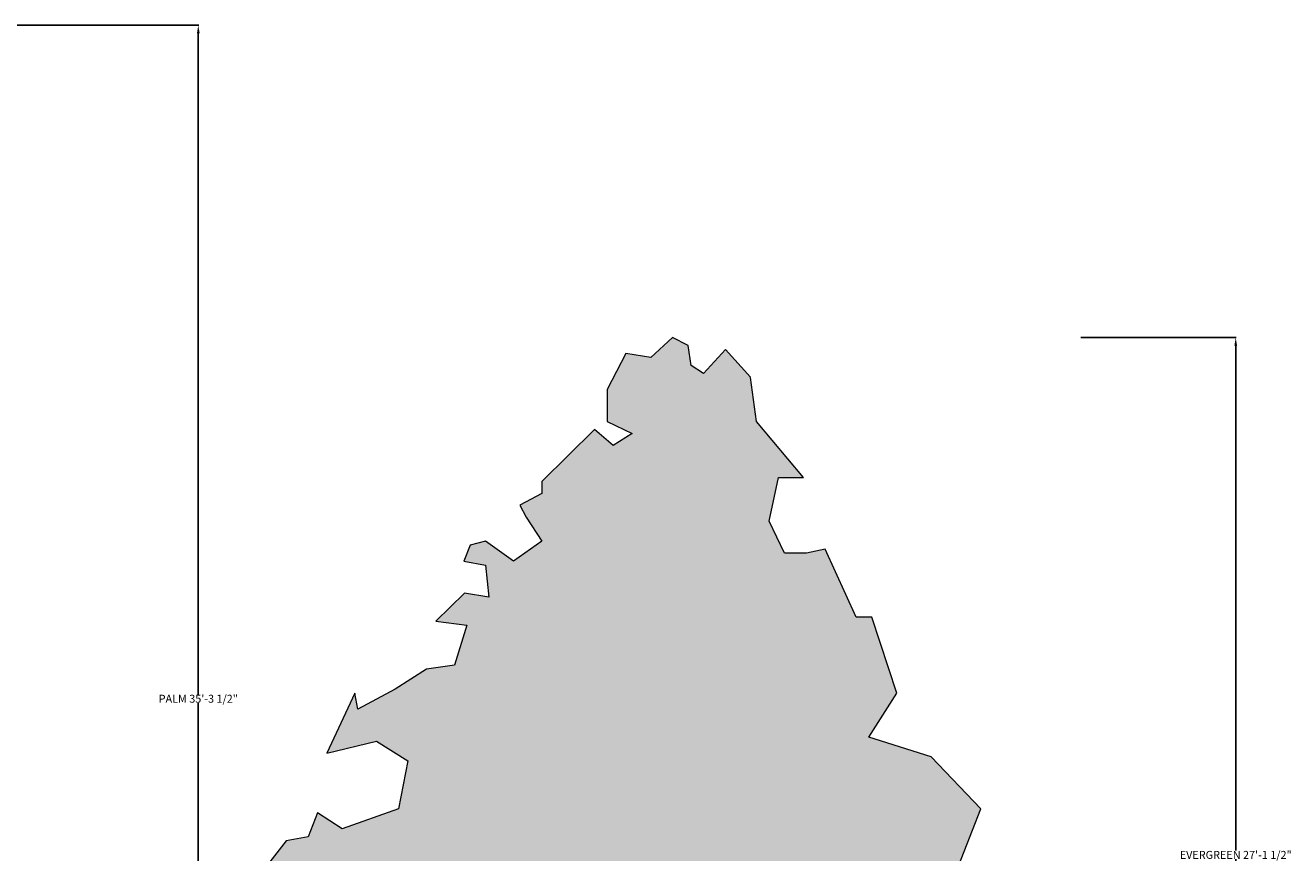
# Model space of a CAD drawing. Units: inches. Extents: x 481 to 2783, y 1975 to 3327.
# Tile 13 of 13: x 2331 to 2729, y 2286 to 2547. Entities that reach past the tile are written whole.
import ezdxf

# ---------------------------------------------------------------- set-up
doc = ezdxf.new("R2010")
doc.units = ezdxf.units.IN
doc.header["$MEASUREMENT"] = 0
doc.layers.add('A-ANNO-DIMS', color=50, linetype='Continuous', lineweight=18)
doc.layers.add('L-PLNT', color=7, linetype='Continuous', lineweight=13)
doc.layers.add('L-PLNT-PATT', color=116, linetype='Continuous', lineweight=13, true_color=0x136734)
doc.styles.get("Standard").update_dxf_attribs({"font": 'arial.ttf'})
doc.dimstyles.get("Standard").update_dxf_attribs({"dimtxt": 2.5, "dimasz": 2.5, "dimexe": 0.18, "dimexo": 0.0625, "dimgap": 0.09, "dimtad": 0, "dimtih": 1, "dimtoh": 1, "dimzin": 0, "dimdsep": 46, "dimlunit": 3, "dimtxsty": 'Standard', "dimcen": 0.09, "dimadec": 0, "dimazin": 0, "dimtfac": 1, "dimtofl": 0, "dimtmove": 0, "dimatfit": 3, "dimfxl": 1, "dimtolj": 1, "dimtzin": 0, "dimarcsym": 0})

# ---------------------------------------------------------------- blocks, each defined once
blk = doc.blocks.new('Tree - type 3 evergreen elevation')
for points in [[(22.0124, 137.721), (18.5475, 141.5624), (15.5282, 138.2446), (13.8028, 139.3505), (13.3714, 142.1153), (11.2148, 143.2214), (8.1954, 140.4564), (4.7447, 141.0094), (2.1567, 136.0326), (2.1567, 131.6088), (5.6074, 129.9499), (3.0193, 128.2909), (0.4313, 130.5029), (-6.9015, 123.3141), (-6.9015, 121.6552), (-9.9208, 119.9963), (-9.0581, 118.3373), (-6.9015, 115.0195), (-10.7835, 112.2546), (-14.6656, 115.0195), (-16.8222, 114.4665), (-17.6849, 112.2546), (-14.6656, 111.7016), (-14.2342, 107.2778), (-17.6065, 107.8307), (-21.5669, 103.9599), (-17.2536, 103.4069), (-18.9789, 97.8771), (-22.8609, 97.3241), (-27.1743, 94.5593), (-32.3504, 91.7944), (-32.7817, 94.0063), (-36.6638, 85.7116), (-29.7624, 87.3705), (-25.449, 84.6056), (-26.743, 77.9699), (-34.507, 75.205), (-37.9578, 77.4169), (-39.2518, 74.099), (-42.2711, 73.5461), (-44.8592, 70.2282), (-47.8786, 66.3574), (-43.9965, 63.0395), (-41.4085, 64.6985), (-44.3346, 59.8898), (-42.2089, 60.1377), (-42.5159, 55.7849), (-49.6039, 46.4502), (-58.2307, 45.8972), (-62.1127, 43.6853), (-68.5828, 36.4966), (-65.9947, 32.0727), (-50.0352, 32.6257), (-47.0159, 30.4138), (-39.6831, 33.7317), (-34.507, 22.6721), (-32.3504, 22.6721), (-22.4296, 34.8376), (-19.4102, 36.4966), (-17.2536, 33.7317), (-17.2536, 29.8608), (-13.8028, 28.7549), (-9.0581, 28.7549), (-7.3328, 32.6257), (-1.7254, 35.3906), (3.8821, 35.9436), (6.4701, 38.1555), (6.9014, 38.7085), (8.1954, 41.4734), (9.9208, 40.3674), (11.2148, 35.9436), (14.2341, 37.6025), (15.0968, 36.4966), (15.9595, 33.7317), (18.9789, 38.7085), (21.9982, 38.7085), (23.2922, 36.4966), (21.9982, 34.2847), (25.4489, 35.3906), (26.743, 33.7317), (29.7623, 35.9436), (32.7817, 34.8376), (38.8204, 28.7549), (41.4084, 27.6489), (43.5651, 25.437), (61.6813, 27.0959), (65.132, 23.7781), (67.7201, 24.884), (60.8186, 33.7317), (60.3873, 37.0495), (62.544, 40.3674), (58.662, 50.874), (56.5053, 50.874), (52.1919, 66.3574), (47.8785, 66.9103), (50.4665, 69.1222), (53.9172, 77.9699), (47.0158, 85.1586), (38.3891, 87.9235), (42.2711, 94.0063)], [(42.2711, 94.0063), (38.8204, 104.5129), (36.6637, 104.5129), (32.3503, 113.9135), (29.7623, 113.3605), (26.743, 113.3605), (24.5862, 117.7844), (25.8802, 123.8671), (29.331, 123.8671), (22.8609, 131.6088), (21.9982, 137.6916)], [(8.1954, 40.3674), (11.2148, 27.6489), (8.1954, 13.8245), (24.5862, 19.9072), (32.7817, 34.2847)], [(-9.9208, 28.2019), (0, 23.2251), (3.4507, 19.9072), (4.7447, 15.4834), (8.6267, 27.0959), (6.4701, 37.6025)], [(34.5071, 33.1787), (27.1743, 18.2483), (9.0581, 10.5066), (7.7641, 3.8708), (8.1954, 0)], [(-12.9401, 28.7549), (-2.588, 22.1191), (0.8626, 17.6953), (1.7253, 11.6125), (0, 0)]]:
    blk.add_lwpolyline(points)
blk = doc.blocks.new('*D56')
at = {"layer": 'A-ANNO-DIMS', "color": 0, "lineweight": -2, "transparency": 16777216}
for p, q in [((2321.97, 2546.55), (2385.65, 2546.55)), ((2385.47, 2544.05), (2385.47, 2336.07)), ((2385.47, 2125.32), (2385.47, 2333.3)), ((2321.97, 2122.82), (2385.65, 2122.82))]:
    blk.add_line(p, q, dxfattribs=at)
at = {"layer": 'A-ANNO-DIMS', "color": 0, "transparency": 16777216}
for points in [[(2385.05, 2544.05), (2385.89, 2544.05), (2385.47, 2546.55)], [(2385.05, 2125.32), (2385.89, 2125.32), (2385.47, 2122.82)]]:
    blk.add_solid(points, dxfattribs=at)
at = {"layer": 'Defpoints', "color": 0, "transparency": 16777216}
for p in [(2321.91, 2546.55), (2385.47, 2546.55), (2321.91, 2122.82)]:
    blk.add_point(p, dxfattribs=at)
at = {"layer": 'A-ANNO-DIMS', "color": 0, "transparency": 16777216, "insert": (2385.47, 2334.69), "char_height": 2.5, "attachment_point": 5}
blk.add_mtext('\\A1;PALM 35\'-3 1/2"', dxfattribs=at)
blk = doc.blocks.new('*D60')
at = {"layer": 'A-ANNO-DIMS', "color": 0, "lineweight": -2, "transparency": 16777216}
for p, q in [((2663.19, 2448.32), (2712.14, 2448.32)), ((2711.96, 2445.82), (2711.96, 2286.95)), ((2711.96, 2125.32), (2711.96, 2284.19)), ((2663.19, 2122.82), (2712.14, 2122.82))]:
    blk.add_line(p, q, dxfattribs=at)
at = {"layer": 'A-ANNO-DIMS', "color": 0, "transparency": 16777216}
for points in [[(2711.54, 2445.82), (2712.37, 2445.82), (2711.96, 2448.32)], [(2711.54, 2125.32), (2712.37, 2125.32), (2711.96, 2122.82)]]:
    blk.add_solid(points, dxfattribs=at)
at = {"layer": 'Defpoints', "color": 0, "transparency": 16777216}
for p in [(2663.13, 2448.32), (2711.96, 2448.32), (2663.13, 2122.82)]:
    blk.add_point(p, dxfattribs=at)
at = {"layer": 'A-ANNO-DIMS', "color": 0, "transparency": 16777216, "insert": (2711.96, 2285.57), "char_height": 2.5, "attachment_point": 5}
blk.add_mtext('\\A1;EVERGREEN 27\'-1 1/2"', dxfattribs=at)

msp = doc.modelspace()

# ---------------------------------------------------------------- hatches: boundary and pattern name
at = {"layer": 'L-PLNT-PATT'}
msp.add_hatch(color=256, dxfattribs=at).paths.add_polyline_path([(2476.873, 2366.633), (2469.209, 2367.89), (2460.208, 2359.093), (2470.011, 2357.836), (2466.089, 2345.268), (2457.267, 2344.011), (2447.464, 2337.728), (2435.7, 2331.444), (2434.72, 2336.471), (2425.897, 2317.619), (2441.582, 2321.389), (2451.385, 2315.106), (2448.444, 2300.025), (2430.798, 2293.741), (2422.956, 2298.768), (2420.015, 2291.227), (2413.153, 2289.97), (2407.271, 2282.43), (2400.408, 2273.633), (2409.231, 2266.092), (2415.113, 2269.862), (2408.463, 2258.933), (2413.294, 2259.497), (2412.596, 2249.604), (2396.487, 2228.389), (2376.881, 2227.132), (2368.058, 2222.105), (2353.354, 2205.767), (2359.236, 2195.713), (2395.507, 2196.97), (2402.369, 2191.943), (2419.035, 2199.483), (2430.798, 2174.348), (2435.7, 2174.348), (2458.247, 2201.997), (2465.109, 2205.767), (2470.011, 2199.483), (2470.011, 2190.686), (2477.853, 2188.172), (2488.637, 2188.172), (2492.558, 2196.97), (2505.302, 2203.254), (2518.046, 2204.51), (2523.928, 2209.537), (2524.908, 2210.794), (2527.849, 2217.078), (2531.77, 2214.564), (2534.711, 2204.51), (2541.573, 2208.281), (2543.534, 2205.767), (2545.495, 2199.483), (2552.357, 2210.794), (2559.219, 2210.794), (2562.16, 2205.767), (2559.219, 2200.74), (2567.062, 2203.254), (2570.003, 2199.483), (2576.865, 2204.51), (2583.727, 2201.997), (2597.451, 2188.172), (2603.333, 2185.659), (2608.235, 2180.632), (2649.408, 2184.402), (2657.25, 2176.862), (2663.132, 2179.375), (2647.447, 2199.483), (2646.467, 2207.024), (2651.368, 2214.564), (2642.546, 2238.443), (2637.644, 2238.443), (2627.841, 2273.633), (2618.038, 2274.889), (2623.92, 2279.916), (2631.762, 2300.025), (2616.077, 2316.362), (2596.471, 2322.646), (2605.294, 2336.471), (2597.451, 2360.349), (2592.55, 2360.349), (2582.746, 2381.714), (2576.865, 2380.458), (2570.003, 2380.458), (2565.101, 2390.512), (2568.042, 2404.336), (2575.884, 2404.336), (2561.18, 2421.931), (2559.202, 2435.877), (2551.377, 2444.553), (2544.515, 2437.012), (2540.593, 2439.526), (2539.613, 2445.809), (2534.711, 2448.323), (2527.849, 2442.039), (2520.007, 2443.296), (2514.125, 2431.985), (2514.125, 2421.931), (2521.967, 2418.161), (2516.085, 2414.39), (2510.203, 2419.417), (2493.538, 2403.079), (2493.538, 2399.309), (2486.676, 2395.539), (2488.637, 2391.768), (2493.538, 2384.228), (2484.715, 2377.944), (2475.892, 2384.228), (2470.991, 2382.971), (2469.03, 2377.944), (2475.892, 2376.687)])

# ---------------------------------------------------------------- block references
at = {"layer": 'L-PLNT', "xscale": 2.272722171462171, "yscale": 2.272722171462171, "zscale": 2.272722171462171}
msp.add_blockref('Tree - type 3 evergreen elevation', (2509.223, 2122.821), dxfattribs=at)

# ---------------------------------------------------------------- dimensions: what is measured, and where the dimension line sits
at = {"layer": 'A-ANNO-DIMS'}
for base, p1, p2, text, picture, middle in [((2385.469, 2546.553), (2321.909, 2122.821), (2321.909, 2546.553), 'PALM <>', '*D56', (2385.469, 2334.687)), ((2711.958, 2448.323), (2663.132, 2122.821), (2663.132, 2448.323), 'EVERGREEN <>', '*D60', (2711.958, 2285.572))]:
    dim = msp.add_linear_dim(base=base, p1=p1, p2=p2, angle=90, text=text, dimstyle='Standard', override={"dimdec": 1, "dimlfac": 1, "dimrnd": 0, "dimzin": 1, "dimdsep": 46, "dimlunit": 4, "dimfrac": 2}, dxfattribs=at)
    dim.commit()
    dim.dimension.update_dxf_attribs({"geometry": picture, "text_midpoint": middle})

doc.saveas('drawing.dxf')
